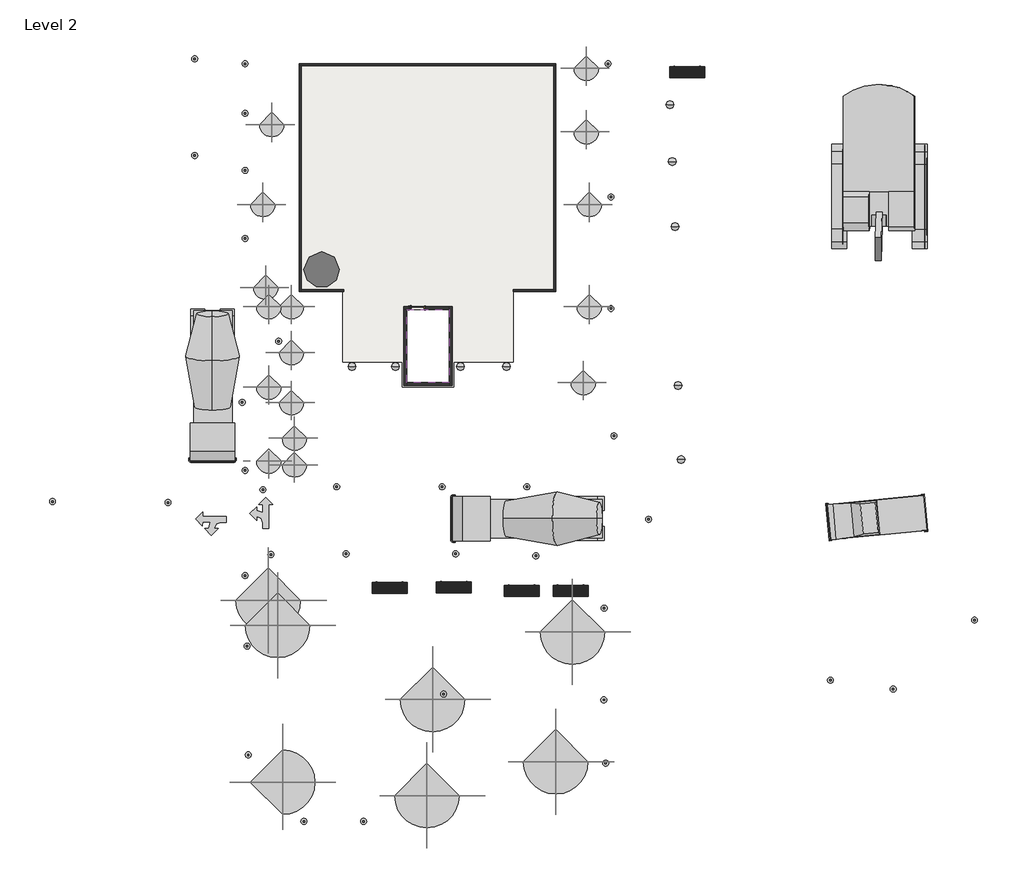
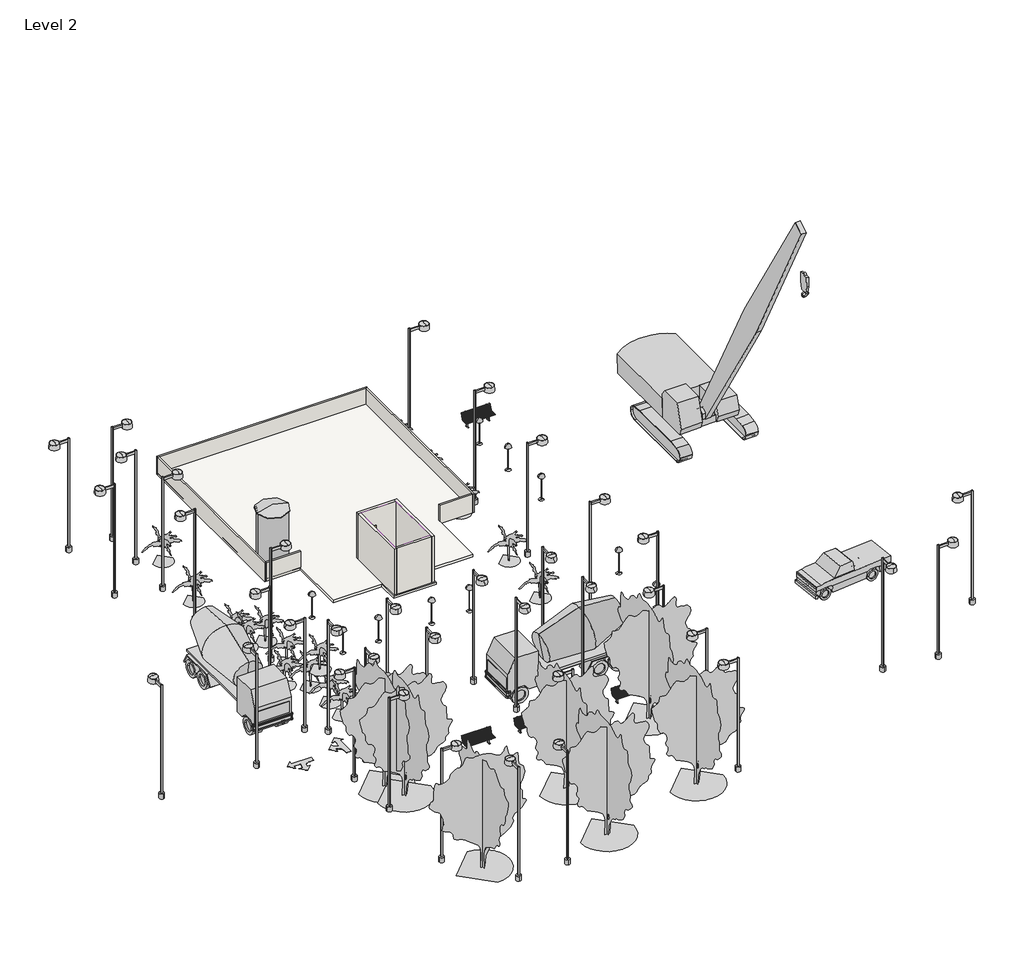
# One storey, incomplete: 46 light fixtures, 34 geographic elements, 9 walls, 1 covering, 1 door, 1 proxy, 1 slab.
"""IFC4 building model written with IfcOpenShell, lengths in millimetres."""

from ifc_helpers import new_model, si_unit, frame, origin, place, context, project, spatial, polyline, outline, extrude, faceted_brep, transform, mapped, element, save
from components import m_watertank_water_tank_eee2c874, door_ef1582a9, geographic_element_33b6fea6, m_concrete_truck_concrete_truck_8dc9909d, m_construction_crane_c1d51077, m_park_bench_1800mm_81f1f144, m_rpc_tree_tropical_australian_tree_fern_1_8_meters_0203a3dd, m_truck_pick_up_pick_up_truck_f485962c, rpc_tree_deciduous_honey_locust_25_cc46a1f1, m_floor_lamp_hemispheric_100w_277v_4a08ccbb, m_street_light_standard_400w_halogen_120v_204dbcbb

model = new_model("IFC4")

# Units and contexts
model_context = context("Model", 3, world=origin())
ifc_project = project(units=[si_unit("LENGTHUNIT", "METRE", prefix="MILLI")], contexts=[model_context])

# Site, building, storey
site = spatial("IfcSite", under=ifc_project)
building = spatial("IfcBuilding", under=site)
storey = spatial("IfcBuildingStorey", under=building, Name="Level 2", Elevation=3200.4)

# Proxy
placement = place(None, origin())
m_watertank_water_tank_shape = m_watertank_water_tank_eee2c874(model_context)
element("IfcBuildingElementProxy", 1, Name="M_WaterTank : Water Tank", ObjectType="M_WaterTank : Water Tank", at=placement, inside=storey, context=model_context, shape_type="MappedRepresentation", body=[
    mapped(m_watertank_water_tank_shape, transform((-12398.6299582, 9055.036641, 3352.8), x_axis=(1.0, 0.0, 0.0), y_axis=(0.0, 1.0, 0.0), z_axis=(0.0, 0.0, 1.0))),
])

# Covering
element("IfcCovering", 2, ObjectType="2' x 4' ACT System", at=placement, inside=storey, context=model_context, shape_type="SweptSolid", body=[
    extrude(outline(polyline([(-8032.1581554, 6997.036641), (-5822.3581554, 6997.036641), (-5822.3581554, 3237.836641), (-8032.1581554, 3237.836641), (-8032.1581554, 6997.036641)])), frame((0.0, 0.0, 6400.8), z_axis=(0.0, 0.0, 1.0), x_axis=(1.0, 0.0, 0.0)), (0.0, 0.0, 1.0), 57.15),
])

# Door
door_shape = door_ef1582a9(model_context)
element("IfcDoor", 3, ObjectType="M_Door-Interior-Single-6_Panel-Wood : 2'5\"", at=placement, inside=storey, context=model_context, shape_type="MappedRepresentation", body=[
    mapped(door_shape, transform((-7498.7581554, 7076.411641, 3352.8), x_axis=(1.0, 0.0, 0.0), y_axis=(0.0, 1.0, 0.0), z_axis=(0.0, 0.0, 1.0))),
])

# Geographic elements
geographic_element_shape = geographic_element_33b6fea6(model_context)
element("IfcGeographicElement", 4, at=placement, inside=storey, context=model_context, shape_type="MappedRepresentation", body=[
    mapped(geographic_element_shape, transform((-17303.3787549, -3805.4849597, -152.4), x_axis=(0.016862452734669187, 0.9998578187361297, 0.0), y_axis=(-0.9998578187361297, 0.016862452734669187, 0.0), z_axis=(0.0, 0.0, 1.0))),
])
element("IfcGeographicElement", 5, at=placement, inside=storey, context=model_context, shape_type="MappedRepresentation", body=[
    mapped(geographic_element_shape, transform((-15269.4299582, -4255.163359, -152.4), x_axis=(1.0, 0.0, 0.0), y_axis=(0.0, 1.0, 0.0), z_axis=(0.0, 0.0, 1.0))),
])
m_concrete_truck_concrete_truck_shape = m_concrete_truck_concrete_truck_8dc9909d(model_context)
element("IfcGeographicElement", 6, ObjectType="M_Concrete Truck : Concrete Truck", at=placement, inside=storey, context=model_context, shape_type="MappedRepresentation", body=[
    mapped(m_concrete_truck_concrete_truck_shape, transform((-17968.6684197, 3155.7751025, -152.4), x_axis=(1.0, 0.0, 0.0), y_axis=(0.0, 1.0, 0.0), z_axis=(0.0, 0.0, 1.0))),
])
element("IfcGeographicElement", 7, ObjectType="M_Concrete Truck : Concrete Truck", at=placement, inside=storey, context=model_context, shape_type="MappedRepresentation", body=[
    mapped(m_concrete_truck_concrete_truck_shape, transform((-1737.0914966, -3803.8248975, -152.4), x_axis=(0.0, -1.0, 0.0), y_axis=(1.0, 0.0, 0.0), z_axis=(0.0, 0.0, 1.0))),
])
m_construction_crane_shape = m_construction_crane_c1d51077(model_context)
element("IfcGeographicElement", 8, ObjectType="M_Construction Crane", at=placement, inside=storey, context=model_context, shape_type="MappedRepresentation", body=[
    mapped(m_construction_crane_shape, transform((21981.1338705, 15716.0751025, 120.4025575), x_axis=(0.9998666340647555, 0.0, 0.016331383407914204), y_axis=(0.0, 1.0, 0.0), z_axis=(-0.016331383407914204, 0.0, 0.9998666340647555))),
])
m_park_bench_1800mm_shape = m_park_bench_1800mm_81f1f144(model_context)
element("IfcGeographicElement", 9, ObjectType="M_Park Bench : 1800mm", at=placement, inside=storey, context=model_context, shape_type="MappedRepresentation", body=[
    mapped(m_park_bench_1800mm_shape, transform((6396.7700418, 19239.836641, -134.1456114), x_axis=(1.0, 0.0, 0.0), y_axis=(0.0, 1.0, 0.0), z_axis=(0.0, 0.0, 1.0))),
])
element("IfcGeographicElement", 10, ObjectType="M_Park Bench : 1800mm", at=placement, inside=storey, context=model_context, shape_type="MappedRepresentation", body=[
    mapped(m_park_bench_1800mm_shape, transform((402.3700418, -7455.563359, -152.4), x_axis=(1.0, 0.0, 0.0), y_axis=(0.0, 1.0, 0.0), z_axis=(0.0, 0.0, 1.0))),
])
element("IfcGeographicElement", 11, ObjectType="M_Park Bench : 1800mm", at=placement, inside=storey, context=model_context, shape_type="MappedRepresentation", body=[
    mapped(m_park_bench_1800mm_shape, transform((-2112.2299582, -7455.563359, -152.4), x_axis=(1.0, 0.0, 0.0), y_axis=(0.0, 1.0, 0.0), z_axis=(0.0, 0.0, 1.0))),
])
element("IfcGeographicElement", 12, ObjectType="M_Park Bench : 1800mm", at=placement, inside=storey, context=model_context, shape_type="MappedRepresentation", body=[
    mapped(m_park_bench_1800mm_shape, transform((-5593.7581554, -7257.9919216, -152.4), x_axis=(1.0, 0.0, 0.0), y_axis=(0.0, 1.0, 0.0), z_axis=(0.0, 0.0, 1.0))),
])
element("IfcGeographicElement", 13, ObjectType="M_Park Bench : 1800mm", at=placement, inside=storey, context=model_context, shape_type="MappedRepresentation", body=[
    mapped(m_park_bench_1800mm_shape, transform((-8906.7299582, -7303.163359, -152.4), x_axis=(1.0, 0.0, 0.0), y_axis=(0.0, 1.0, 0.0), z_axis=(0.0, 0.0, 1.0))),
])
m_rpc_tree_tropical_australian_tree_fern_1_8_meters_shape = m_rpc_tree_tropical_australian_tree_fern_1_8_meters_0203a3dd(model_context)
element("IfcGeographicElement", 14, ObjectType="M_RPC Tree - Tropical : Australian Tree Fern - 1.8 Meters", at=placement, inside=storey, context=model_context, shape_type="MappedRepresentation", body=[
    mapped(m_rpc_tree_tropical_australian_tree_fern_1_8_meters_shape, transform((1214.9733707, 19417.636641, -152.4), x_axis=(1.0, 0.0, 0.0), y_axis=(0.0, 1.0, 0.0), z_axis=(0.0, 0.0, 1.0))),
])
element("IfcGeographicElement", 15, ObjectType="M_RPC Tree - Tropical : Australian Tree Fern - 1.8 Meters", at=placement, inside=storey, context=model_context, shape_type="MappedRepresentation", body=[
    mapped(m_rpc_tree_tropical_australian_tree_fern_1_8_meters_shape, transform((1214.9733707, 16141.036641, -152.4), x_axis=(1.0, 0.0, 0.0), y_axis=(0.0, 1.0, 0.0), z_axis=(0.0, 0.0, 1.0))),
])
element("IfcGeographicElement", 16, ObjectType="M_RPC Tree - Tropical : Australian Tree Fern - 1.8 Meters", at=placement, inside=storey, context=model_context, shape_type="MappedRepresentation", body=[
    mapped(m_rpc_tree_tropical_australian_tree_fern_1_8_meters_shape, transform((1367.3733707, 12407.236641, -152.4), x_axis=(1.0, 0.0, 0.0), y_axis=(0.0, 1.0, 0.0), z_axis=(0.0, 0.0, 1.0))),
])
element("IfcGeographicElement", 17, ObjectType="M_RPC Tree - Tropical : Australian Tree Fern - 1.8 Meters", at=placement, inside=storey, context=model_context, shape_type="MappedRepresentation", body=[
    mapped(m_rpc_tree_tropical_australian_tree_fern_1_8_meters_shape, transform((1367.3733707, 7149.436641, -152.4), x_axis=(1.0, 0.0, 0.0), y_axis=(0.0, 1.0, 0.0), z_axis=(0.0, 0.0, 1.0))),
])
element("IfcGeographicElement", 18, ObjectType="M_RPC Tree - Tropical : Australian Tree Fern - 1.8 Meters", at=placement, inside=storey, context=model_context, shape_type="MappedRepresentation", body=[
    mapped(m_rpc_tree_tropical_australian_tree_fern_1_8_meters_shape, transform((1062.5733707, 3237.836641, -152.4), x_axis=(1.0, 0.0, 0.0), y_axis=(0.0, 1.0, 0.0), z_axis=(0.0, 0.0, 1.0))),
])
element("IfcGeographicElement", 19, ObjectType="M_RPC Tree - Tropical : Australian Tree Fern - 1.8 Meters", at=placement, inside=storey, context=model_context, shape_type="MappedRepresentation", body=[
    mapped(m_rpc_tree_tropical_australian_tree_fern_1_8_meters_shape, transform((-15117.2266293, 3009.236641, -152.4), x_axis=(1.0, 0.0, 0.0), y_axis=(0.0, 1.0, 0.0), z_axis=(0.0, 0.0, 1.0))),
])
element("IfcGeographicElement", 20, ObjectType="M_RPC Tree - Tropical : Australian Tree Fern - 1.8 Meters", at=placement, inside=storey, context=model_context, shape_type="MappedRepresentation", body=[
    mapped(m_rpc_tree_tropical_australian_tree_fern_1_8_meters_shape, transform((-15117.2266293, 7149.436641, -152.4), x_axis=(1.0, 0.0, 0.0), y_axis=(0.0, 1.0, 0.0), z_axis=(0.0, 0.0, 1.0))),
])
element("IfcGeographicElement", 21, ObjectType="M_RPC Tree - Tropical : Australian Tree Fern - 1.8 Meters", at=placement, inside=storey, context=model_context, shape_type="MappedRepresentation", body=[
    mapped(m_rpc_tree_tropical_australian_tree_fern_1_8_meters_shape, transform((-14964.8266293, 16522.036641, -152.4), x_axis=(1.0, 0.0, 0.0), y_axis=(0.0, 1.0, 0.0), z_axis=(0.0, 0.0, 1.0))),
])
element("IfcGeographicElement", 22, ObjectType="M_RPC Tree - Tropical : Australian Tree Fern - 1.8 Meters", at=placement, inside=storey, context=model_context, shape_type="MappedRepresentation", body=[
    mapped(m_rpc_tree_tropical_australian_tree_fern_1_8_meters_shape, transform((-15117.2266293, -800.763359, 3200.4), x_axis=(1.0, 0.0, 0.0), y_axis=(0.0, 1.0, 0.0), z_axis=(0.0, 0.0, 1.0))),
])
element("IfcGeographicElement", 23, ObjectType="M_RPC Tree - Tropical : Australian Tree Fern - 1.8 Meters", at=placement, inside=storey, context=model_context, shape_type="MappedRepresentation", body=[
    mapped(m_rpc_tree_tropical_australian_tree_fern_1_8_meters_shape, transform((-15422.0266293, 12407.236641, -152.4), x_axis=(1.0, 0.0, 0.0), y_axis=(0.0, 1.0, 0.0), z_axis=(0.0, 0.0, 1.0))),
])
element("IfcGeographicElement", 24, ObjectType="M_RPC Tree - Tropical : Australian Tree Fern - 1.8 Meters", at=placement, inside=storey, context=model_context, shape_type="MappedRepresentation", body=[
    mapped(m_rpc_tree_tropical_australian_tree_fern_1_8_meters_shape, transform((-15269.6266293, 8140.036641, -152.4), x_axis=(1.0, 0.0, 0.0), y_axis=(0.0, 1.0, 0.0), z_axis=(0.0, 0.0, 1.0))),
])
element("IfcGeographicElement", 25, ObjectType="M_RPC Tree - Tropical : Australian Tree Fern - 1.8 Meters", at=placement, inside=storey, context=model_context, shape_type="MappedRepresentation", body=[
    mapped(m_rpc_tree_tropical_australian_tree_fern_1_8_meters_shape, transform((-13948.8266293, 7149.436641, -152.4), x_axis=(1.0, 0.0, 0.0), y_axis=(0.0, 1.0, 0.0), z_axis=(0.0, 0.0, 1.0))),
])
element("IfcGeographicElement", 26, ObjectType="M_RPC Tree - Tropical : Australian Tree Fern - 1.8 Meters", at=placement, inside=storey, context=model_context, shape_type="MappedRepresentation", body=[
    mapped(m_rpc_tree_tropical_australian_tree_fern_1_8_meters_shape, transform((-13948.8266293, 4787.236641, -152.4), x_axis=(1.0, 0.0, 0.0), y_axis=(0.0, 1.0, 0.0), z_axis=(0.0, 0.0, 1.0))),
])
element("IfcGeographicElement", 27, ObjectType="M_RPC Tree - Tropical : Australian Tree Fern - 1.8 Meters", at=placement, inside=storey, context=model_context, shape_type="MappedRepresentation", body=[
    mapped(m_rpc_tree_tropical_australian_tree_fern_1_8_meters_shape, transform((-13948.8266293, 2209.136641, -152.4), x_axis=(1.0, 0.0, 0.0), y_axis=(0.0, 1.0, 0.0), z_axis=(0.0, 0.0, 1.0))),
])
element("IfcGeographicElement", 28, ObjectType="M_RPC Tree - Tropical : Australian Tree Fern - 1.8 Meters", at=placement, inside=storey, context=model_context, shape_type="MappedRepresentation", body=[
    mapped(m_rpc_tree_tropical_australian_tree_fern_1_8_meters_shape, transform((-13796.4266293, 380.336641, -152.4), x_axis=(1.0, 0.0, 0.0), y_axis=(0.0, 1.0, 0.0), z_axis=(0.0, 0.0, 1.0))),
])
element("IfcGeographicElement", 29, ObjectType="M_RPC Tree - Tropical : Australian Tree Fern - 1.8 Meters", at=placement, inside=storey, context=model_context, shape_type="MappedRepresentation", body=[
    mapped(m_rpc_tree_tropical_australian_tree_fern_1_8_meters_shape, transform((-13796.4266293, -991.263359, -152.4), x_axis=(1.0, 0.0, 0.0), y_axis=(0.0, 1.0, 0.0), z_axis=(0.0, 0.0, 1.0))),
])
m_truck_pick_up_pick_up_truck_shape = m_truck_pick_up_pick_up_truck_f485962c(model_context)
element("IfcGeographicElement", 30, ObjectType="M_Truck - Pick-Up : Pick-Up Truck", at=placement, inside=storey, context=model_context, shape_type="MappedRepresentation", body=[
    mapped(m_truck_pick_up_pick_up_truck_shape, transform((15628.1031197, -3722.1387124, -152.4), x_axis=(0.0952515948864838, -0.9954532302783397, 0.0), y_axis=(0.9954532302783397, 0.0952515948864838, 0.0), z_axis=(0.0, 0.0, 1.0))),
])
rpc_tree_deciduous_honey_locust_25_shape = rpc_tree_deciduous_honey_locust_25_cc46a1f1(model_context)
element("IfcGeographicElement", 31, ObjectType="RPC Tree - Deciduous : Honey Locust - 25'", at=placement, inside=storey, context=model_context, shape_type="MappedRepresentation", body=[
    mapped(rpc_tree_deciduous_honey_locust_25_shape, transform((503.9700418, -9597.0505555, -152.4), x_axis=(1.0, 0.0, 0.0), y_axis=(0.0, 1.0, 0.0), z_axis=(0.0, 0.0, 1.0))),
])
element("IfcGeographicElement", 32, ObjectType="RPC Tree - Deciduous : Honey Locust - 25'", at=placement, inside=storey, context=model_context, shape_type="MappedRepresentation", body=[
    mapped(rpc_tree_deciduous_honey_locust_25_shape, transform((-15145.9347705, -7965.3174698, -152.4), x_axis=(1.0, 0.0, 0.0), y_axis=(0.0, 1.0, 0.0), z_axis=(0.0, 0.0, 1.0))),
])
element("IfcGeographicElement", 33, ObjectType="RPC Tree - Deciduous : Honey Locust - 25'", at=placement, inside=storey, context=model_context, shape_type="MappedRepresentation", body=[
    mapped(rpc_tree_deciduous_honey_locust_25_shape, transform((-6694.0035501, -13068.9779282, -152.4), x_axis=(1.0, 0.0, 0.0), y_axis=(0.0, 1.0, 0.0), z_axis=(0.0, 0.0, 1.0))),
])
element("IfcGeographicElement", 34, ObjectType="RPC Tree - Deciduous : Honey Locust - 25'", at=placement, inside=storey, context=model_context, shape_type="MappedRepresentation", body=[
    mapped(rpc_tree_deciduous_honey_locust_25_shape, transform((-359.6299582, -16269.9199129, -152.4), x_axis=(1.0, 0.0, 0.0), y_axis=(0.0, 1.0, 0.0), z_axis=(0.0, 0.0, 1.0))),
])
element("IfcGeographicElement", 35, ObjectType="RPC Tree - Deciduous : Honey Locust - 25'", at=placement, inside=storey, context=model_context, shape_type="MappedRepresentation", body=[
    mapped(rpc_tree_deciduous_honey_locust_25_shape, transform((-14405.8299582, -17330.8911171, -152.4), x_axis=(0.0, 1.0, 0.0), y_axis=(-1.0, 0.0, 0.0), z_axis=(0.0, 0.0, 1.0))),
])
element("IfcGeographicElement", 36, ObjectType="RPC Tree - Deciduous : Honey Locust - 25'", at=placement, inside=storey, context=model_context, shape_type="MappedRepresentation", body=[
    mapped(rpc_tree_deciduous_honey_locust_25_shape, transform((-14664.2636101, -9251.2975297, -152.4), x_axis=(1.0, 0.0, 0.0), y_axis=(0.0, 1.0, 0.0), z_axis=(0.0, 0.0, 1.0))),
])
element("IfcGeographicElement", 37, ObjectType="RPC Tree - Deciduous : Honey Locust - 25'", at=placement, inside=storey, context=model_context, shape_type="MappedRepresentation", body=[
    mapped(rpc_tree_deciduous_honey_locust_25_shape, transform((-6981.0037801, -18013.7214545, -152.4), x_axis=(1.0, 0.0, 0.0), y_axis=(0.0, 1.0, 0.0), z_axis=(0.0, 0.0, 1.0))),
])

# Light fixtures
m_floor_lamp_hemispheric_100w_277v_shape = m_floor_lamp_hemispheric_100w_277v_4a08ccbb(model_context)
element("IfcLightFixture", 38, ObjectType="M_Floor Lamp - Hemispheric : 100W - 277V", at=placement, inside=storey, context=model_context, shape_type="MappedRepresentation", body=[
    mapped(m_floor_lamp_hemispheric_100w_277v_shape, transform((-8603.6581554, 4063.336641, -152.4), x_axis=(1.0, 0.0, 0.0), y_axis=(0.0, 1.0, 0.0), z_axis=(0.0, 0.0, 1.0))),
])
element("IfcLightFixture", 39, ObjectType="M_Floor Lamp - Hemispheric : 100W - 277V", at=placement, inside=storey, context=model_context, shape_type="MappedRepresentation", body=[
    mapped(m_floor_lamp_hemispheric_100w_277v_shape, transform((-10837.1299582, 4063.336641, -152.4), x_axis=(1.0, 0.0, 0.0), y_axis=(0.0, 1.0, 0.0), z_axis=(0.0, 0.0, 1.0))),
])
element("IfcLightFixture", 40, ObjectType="M_Floor Lamp - Hemispheric : 100W - 277V", at=placement, inside=storey, context=model_context, shape_type="MappedRepresentation", body=[
    mapped(m_floor_lamp_hemispheric_100w_277v_shape, transform((-2899.6299582, 4063.336641, -152.4), x_axis=(1.0, 0.0, 0.0), y_axis=(0.0, 1.0, 0.0), z_axis=(0.0, 0.0, 1.0))),
])
element("IfcLightFixture", 41, ObjectType="M_Floor Lamp - Hemispheric : 100W - 277V", at=placement, inside=storey, context=model_context, shape_type="MappedRepresentation", body=[
    mapped(m_floor_lamp_hemispheric_100w_277v_shape, transform((-5261.8299582, 4063.336641, -152.4), x_axis=(1.0, 0.0, 0.0), y_axis=(0.0, 1.0, 0.0), z_axis=(0.0, 0.0, 1.0))),
])
element("IfcLightFixture", 42, ObjectType="M_Floor Lamp - Hemispheric : 100W - 277V", at=placement, inside=storey, context=model_context, shape_type="MappedRepresentation", body=[
    mapped(m_floor_lamp_hemispheric_100w_277v_shape, transform((-10621.2299582, 7809.836641, -152.4), x_axis=(1.0, 0.0, 0.0), y_axis=(0.0, 1.0, 0.0), z_axis=(0.0, 0.0, 1.0))),
])
element("IfcLightFixture", 43, ObjectType="M_Floor Lamp - Hemispheric : 60W - 120V", at=placement, inside=storey, context=model_context, shape_type="MappedRepresentation", body=[
    mapped(m_floor_lamp_hemispheric_100w_277v_shape, transform((5513.1332848, 17539.0360942, -148.5785469), x_axis=(1.0, 0.0, 0.0), y_axis=(0.0, 1.0, 0.0), z_axis=(0.0, 0.0, 1.0))),
])
element("IfcLightFixture", 44, ObjectType="M_Floor Lamp - Hemispheric : 60W - 120V", at=placement, inside=storey, context=model_context, shape_type="MappedRepresentation", body=[
    mapped(m_floor_lamp_hemispheric_100w_277v_shape, transform((5634.7700418, 14617.036641, -146.5917854), x_axis=(1.0, 0.0, 0.0), y_axis=(0.0, 1.0, 0.0), z_axis=(0.0, 0.0, 1.0))),
])
element("IfcLightFixture", 45, ObjectType="M_Floor Lamp - Hemispheric : 60W - 120V", at=placement, inside=storey, context=model_context, shape_type="MappedRepresentation", body=[
    mapped(m_floor_lamp_hemispheric_100w_277v_shape, transform((5787.1700418, 11264.236641, -144.1025506), x_axis=(1.0, 0.0, 0.0), y_axis=(0.0, 1.0, 0.0), z_axis=(0.0, 0.0, 1.0))),
])
element("IfcLightFixture", 46, ObjectType="M_Floor Lamp - Hemispheric : 60W - 120V", at=placement, inside=storey, context=model_context, shape_type="MappedRepresentation", body=[
    mapped(m_floor_lamp_hemispheric_100w_277v_shape, transform((5939.5700418, 3085.436641, -141.6133158), x_axis=(1.0, 0.0, 0.0), y_axis=(0.0, 1.0, 0.0), z_axis=(0.0, 0.0, 1.0))),
])
element("IfcLightFixture", 47, ObjectType="M_Floor Lamp - Hemispheric : 60W - 120V", at=placement, inside=storey, context=model_context, shape_type="MappedRepresentation", body=[
    mapped(m_floor_lamp_hemispheric_100w_277v_shape, transform((6091.9700418, -724.563359, -145.0919931), x_axis=(1.0, 0.0, 0.0), y_axis=(0.0, 1.0, 0.0), z_axis=(0.0, 0.0, 1.0))),
])
m_street_light_standard_400w_halogen_120v_shape = m_street_light_standard_400w_halogen_120v_204dbcbb(model_context)
element("IfcLightFixture", 48, ObjectType="M_Street Light - Standard : 400W Halogen - 120V", at=placement, inside=storey, context=model_context, shape_type="MappedRepresentation", body=[
    mapped(m_street_light_standard_400w_halogen_120v_shape, transform((2332.7700418, 19646.236641, -152.4), x_axis=(-1.0, 0.0, 0.0), y_axis=(0.0, -1.0, 0.0), z_axis=(0.0, 0.0, 1.0))),
])
element("IfcLightFixture", 49, ObjectType="M_Street Light - Standard : 400W Halogen - 120V", at=placement, inside=storey, context=model_context, shape_type="MappedRepresentation", body=[
    mapped(m_street_light_standard_400w_halogen_120v_shape, transform((2485.1700418, 12788.236641, -152.4), x_axis=(-1.0, 0.0, 0.0), y_axis=(0.0, -1.0, 0.0), z_axis=(0.0, 0.0, 1.0))),
])
element("IfcLightFixture", 50, ObjectType="M_Street Light - Standard : 400W Halogen - 120V", at=placement, inside=storey, context=model_context, shape_type="MappedRepresentation", body=[
    mapped(m_street_light_standard_400w_halogen_120v_shape, transform((2637.5700418, 494.636641, -152.4), x_axis=(-1.0, 0.0, 0.0), y_axis=(0.0, -1.0, 0.0), z_axis=(0.0, 0.0, 1.0))),
])
element("IfcLightFixture", 51, ObjectType="M_Street Light - Standard : 400W Halogen - 120V", at=placement, inside=storey, context=model_context, shape_type="MappedRepresentation", body=[
    mapped(m_street_light_standard_400w_halogen_120v_shape, transform((2485.1700418, 7047.836641, -152.4), x_axis=(-1.0, 0.0, 0.0), y_axis=(0.0, -1.0, 0.0), z_axis=(0.0, 0.0, 1.0))),
])
element("IfcLightFixture", 52, ObjectType="M_Street Light - Standard : 400W Halogen - 120V", at=placement, inside=storey, context=model_context, shape_type="MappedRepresentation", body=[
    mapped(m_street_light_standard_400w_halogen_120v_shape, transform((-15421.8299582, -2273.963359, 0.0), x_axis=(0.0, 1.0, 0.0), y_axis=(-1.0, 0.0, 0.0), z_axis=(0.0, 0.0, 1.0))),
])
element("IfcLightFixture", 53, ObjectType="M_Street Light - Standard : 400W Halogen - 120V", at=placement, inside=storey, context=model_context, shape_type="MappedRepresentation", body=[
    mapped(m_street_light_standard_400w_halogen_120v_shape, transform((-11624.5299582, -2121.563359, 0.0), x_axis=(0.0, 1.0, 0.0), y_axis=(-1.0, 0.0, 0.0), z_axis=(0.0, 0.0, 1.0))),
])
element("IfcLightFixture", 54, ObjectType="M_Street Light - Standard : 400W Halogen - 120V", at=placement, inside=storey, context=model_context, shape_type="MappedRepresentation", body=[
    mapped(m_street_light_standard_400w_halogen_120v_shape, transform((-6203.3581554, -2121.563359, 0.0), x_axis=(0.0, 1.0, 0.0), y_axis=(-1.0, 0.0, 0.0), z_axis=(0.0, 0.0, 1.0))),
])
element("IfcLightFixture", 55, ObjectType="M_Street Light - Standard : 400W Halogen - 120V", at=placement, inside=storey, context=model_context, shape_type="MappedRepresentation", body=[
    mapped(m_street_light_standard_400w_halogen_120v_shape, transform((-1845.5299582, -2121.563359, 0.0), x_axis=(0.0, 1.0, 0.0), y_axis=(-1.0, 0.0, 0.0), z_axis=(0.0, 0.0, 1.0))),
])
element("IfcLightFixture", 56, ObjectType="M_Street Light - Standard : 400W Halogen - 120V", at=placement, inside=storey, context=model_context, shape_type="MappedRepresentation", body=[
    mapped(m_street_light_standard_400w_halogen_120v_shape, transform((-15006.5505126, -5608.7033445, 0.0), x_axis=(0.0, 1.0, 0.0), y_axis=(-1.0, 0.0, 0.0), z_axis=(0.0, 0.0, 1.0))),
])
element("IfcLightFixture", 57, ObjectType="M_Street Light - Standard : 400W Halogen - 120V", at=placement, inside=storey, context=model_context, shape_type="MappedRepresentation", body=[
    mapped(m_street_light_standard_400w_halogen_120v_shape, transform((-11141.9299582, -5575.963359, 0.0), x_axis=(0.0, 1.0, 0.0), y_axis=(-1.0, 0.0, 0.0), z_axis=(0.0, 0.0, 1.0))),
])
element("IfcLightFixture", 58, ObjectType="M_Street Light - Standard : 400W Halogen - 120V", at=placement, inside=storey, context=model_context, shape_type="MappedRepresentation", body=[
    mapped(m_street_light_standard_400w_halogen_120v_shape, transform((-5503.1299582, -5575.963359, 0.0), x_axis=(0.0, 1.0, 0.0), y_axis=(-1.0, 0.0, 0.0), z_axis=(0.0, 0.0, 1.0))),
])
element("IfcLightFixture", 59, ObjectType="M_Street Light - Standard : 400W Halogen - 120V", at=placement, inside=storey, context=model_context, shape_type="MappedRepresentation", body=[
    mapped(m_street_light_standard_400w_halogen_120v_shape, transform((-1383.290395, -5679.9051322, 0.0), x_axis=(0.0, 1.0, 0.0), y_axis=(-1.0, 0.0, 0.0), z_axis=(0.0, 0.0, 1.0))),
])
element("IfcLightFixture", 60, ObjectType="M_Street Light - Standard : 400W Halogen - 120V", at=placement, inside=storey, context=model_context, shape_type="MappedRepresentation", body=[
    mapped(m_street_light_standard_400w_halogen_120v_shape, transform((2129.5700418, -8369.963359, -152.4), x_axis=(1.0, 0.0, 0.0), y_axis=(0.0, 1.0, 0.0), z_axis=(0.0, 0.0, 1.0))),
])
element("IfcLightFixture", 61, ObjectType="M_Street Light - Standard : 400W Halogen - 120V", at=placement, inside=storey, context=model_context, shape_type="MappedRepresentation", body=[
    mapped(m_street_light_standard_400w_halogen_120v_shape, transform((2117.2753399, -13089.3237573, -152.4), x_axis=(1.0, 0.0, 0.0), y_axis=(0.0, 1.0, 0.0), z_axis=(0.0, 0.0, 1.0))),
])
element("IfcLightFixture", 62, ObjectType="M_Street Light - Standard : 400W Halogen - 120V", at=placement, inside=storey, context=model_context, shape_type="MappedRepresentation", body=[
    mapped(m_street_light_standard_400w_halogen_120v_shape, transform((2210.8272988, -16350.1092884, -152.4), x_axis=(1.0, 0.0, 0.0), y_axis=(0.0, 1.0, 0.0), z_axis=(0.0, 0.0, 1.0))),
])
element("IfcLightFixture", 63, ObjectType="M_Street Light - Standard : 400W Halogen - 120V", at=placement, inside=storey, context=model_context, shape_type="MappedRepresentation", body=[
    mapped(m_street_light_standard_400w_halogen_120v_shape, transform((13769.7128986, -12075.4373856, -152.4), x_axis=(0.0, 1.0, 0.0), y_axis=(-1.0, 0.0, 0.0), z_axis=(0.0, 0.0, 1.0))),
])
element("IfcLightFixture", 64, ObjectType="M_Street Light - Standard : 400W Halogen - 120V", at=placement, inside=storey, context=model_context, shape_type="MappedRepresentation", body=[
    mapped(m_street_light_standard_400w_halogen_120v_shape, transform((16994.3658729, -12532.6373856, -152.4), x_axis=(-1.0, 0.0, 0.0), y_axis=(0.0, -1.0, 0.0), z_axis=(0.0, 0.0, 1.0))),
])
element("IfcLightFixture", 65, ObjectType="M_Street Light - Standard : 400W Halogen - 120V", at=placement, inside=storey, context=model_context, shape_type="MappedRepresentation", body=[
    mapped(m_street_light_standard_400w_halogen_120v_shape, transform((21179.5700418, -8979.563359, -152.4), x_axis=(1.0, 0.0, 0.0), y_axis=(0.0, 1.0, 0.0), z_axis=(0.0, 0.0, 1.0))),
])
element("IfcLightFixture", 66, ObjectType="M_Street Light - Standard : 400W Halogen - 120V", at=placement, inside=storey, context=model_context, shape_type="MappedRepresentation", body=[
    mapped(m_street_light_standard_400w_halogen_120v_shape, transform((4415.5700418, -3797.963359, -152.4), x_axis=(1.0, 0.0, 0.0), y_axis=(0.0, 1.0, 0.0), z_axis=(0.0, 0.0, 1.0))),
])
element("IfcLightFixture", 67, ObjectType="M_Street Light - Standard : 400W Halogen - 120V", at=placement, inside=storey, context=model_context, shape_type="MappedRepresentation", body=[
    mapped(m_street_light_standard_400w_halogen_120v_shape, transform((-16232.9652381, -10322.7398887, 0.0), x_axis=(-1.0, 0.0, 0.0), y_axis=(0.0, -1.0, 0.0), z_axis=(0.0, 0.0, 1.0))),
])
element("IfcLightFixture", 68, ObjectType="M_Street Light - Standard : 400W Halogen - 120V", at=placement, inside=storey, context=model_context, shape_type="MappedRepresentation", body=[
    mapped(m_street_light_standard_400w_halogen_120v_shape, transform((-16172.8526522, -15918.8024863, 0.0), x_axis=(-1.0, 0.0, 0.0), y_axis=(0.0, -1.0, 0.0), z_axis=(0.0, 0.0, 1.0))),
])
element("IfcLightFixture", 69, ObjectType="M_Street Light - Standard : 400W Halogen - 120V", at=placement, inside=storey, context=model_context, shape_type="MappedRepresentation", body=[
    mapped(m_street_light_standard_400w_halogen_120v_shape, transform((-16336.2299582, 19646.236641, -152.4), x_axis=(-1.0, 0.0, 0.0), y_axis=(0.0, -1.0, 0.0), z_axis=(0.0, 0.0, 1.0))),
])
element("IfcLightFixture", 70, ObjectType="M_Street Light - Standard : 400W Halogen - 120V", at=placement, inside=storey, context=model_context, shape_type="MappedRepresentation", body=[
    mapped(m_street_light_standard_400w_halogen_120v_shape, transform((-16336.2299582, 17093.536641, -152.4), x_axis=(1.0, 0.0, 0.0), y_axis=(0.0, 1.0, 0.0), z_axis=(0.0, 0.0, 1.0))),
])
element("IfcLightFixture", 71, ObjectType="M_Street Light - Standard : 400W Halogen - 120V", at=placement, inside=storey, context=model_context, shape_type="MappedRepresentation", body=[
    mapped(m_street_light_standard_400w_halogen_120v_shape, transform((-16336.2299582, 14159.836641, -152.4), x_axis=(-1.0, 0.0, 0.0), y_axis=(0.0, -1.0, 0.0), z_axis=(0.0, 0.0, 1.0))),
])
element("IfcLightFixture", 72, ObjectType="M_Street Light - Standard : 400W Halogen - 120V", at=placement, inside=storey, context=model_context, shape_type="MappedRepresentation", body=[
    mapped(m_street_light_standard_400w_halogen_120v_shape, transform((-16336.2299582, 10654.636641, -152.4), x_axis=(1.0, 0.0, 0.0), y_axis=(0.0, 1.0, 0.0), z_axis=(0.0, 0.0, 1.0))),
])
element("IfcLightFixture", 73, ObjectType="M_Street Light - Standard : 400W Halogen - 120V", at=placement, inside=storey, context=model_context, shape_type="MappedRepresentation", body=[
    mapped(m_street_light_standard_400w_halogen_120v_shape, transform((-18927.0299582, 19900.236641, -152.3997054), x_axis=(1.0, 0.0, 0.0), y_axis=(0.0, 1.0, 0.0), z_axis=(0.0, 0.0, 1.0))),
])
element("IfcLightFixture", 74, ObjectType="M_Street Light - Standard : 400W Halogen - 120V", at=placement, inside=storey, context=model_context, shape_type="MappedRepresentation", body=[
    mapped(m_street_light_standard_400w_halogen_120v_shape, transform((-18927.0299582, 14921.836641, -152.3997054), x_axis=(1.0, 0.0, 0.0), y_axis=(0.0, 1.0, 0.0), z_axis=(0.0, 0.0, 1.0))),
])
element("IfcLightFixture", 75, ObjectType="M_Street Light - Standard : 400W Halogen - 120V", at=placement, inside=storey, context=model_context, shape_type="MappedRepresentation", body=[
    mapped(m_street_light_standard_400w_halogen_120v_shape, transform((-26242.2299582, -2883.563359, -152.4), x_axis=(0.0, -1.0, 0.0), y_axis=(1.0, 0.0, 0.0), z_axis=(0.0, 0.0, 1.0))),
])
element("IfcLightFixture", 76, ObjectType="M_Street Light - Standard : 400W Halogen - 120V", at=placement, inside=storey, context=model_context, shape_type="MappedRepresentation", body=[
    mapped(m_street_light_standard_400w_halogen_120v_shape, transform((-20298.6299582, -2934.363359, -152.3997054), x_axis=(0.0, -1.0, 0.0), y_axis=(1.0, 0.0, 0.0), z_axis=(0.0, 0.0, 1.0))),
])
element("IfcLightFixture", 77, ObjectType="M_Street Light - Standard : 400W Halogen - 480V", at=placement, inside=storey, context=model_context, shape_type="MappedRepresentation", body=[
    mapped(m_street_light_standard_400w_halogen_120v_shape, transform((-16336.2299582, -6693.563359, -152.4), x_axis=(1.0, 0.0, 0.0), y_axis=(0.0, 1.0, 0.0), z_axis=(0.0, 0.0, 1.0))),
])
element("IfcLightFixture", 78, ObjectType="M_Street Light - Standard : 400W Halogen - 480V", at=placement, inside=storey, context=model_context, shape_type="MappedRepresentation", body=[
    mapped(m_street_light_standard_400w_halogen_120v_shape, transform((-10240.2299582, -19342.763359, -152.4), x_axis=(0.0, -1.0, 0.0), y_axis=(1.0, 0.0, 0.0), z_axis=(0.0, 0.0, 1.0))),
])
element("IfcLightFixture", 79, ObjectType="M_Street Light - Standard : 400W Halogen - 480V", at=placement, inside=storey, context=model_context, shape_type="MappedRepresentation", body=[
    mapped(m_street_light_standard_400w_halogen_120v_shape, transform((-13313.6299582, -19342.763359, -152.4), x_axis=(0.0, -1.0, 0.0), y_axis=(1.0, 0.0, 0.0), z_axis=(0.0, 0.0, 1.0))),
])
element("IfcLightFixture", 80, ObjectType="M_Street Light - Standard : 400W Halogen - 480V", at=placement, inside=storey, context=model_context, shape_type="MappedRepresentation", body=[
    mapped(m_street_light_standard_400w_halogen_120v_shape, transform((-6125.4299582, -12789.563359, -152.4), x_axis=(1.0, 0.0, 0.0), y_axis=(0.0, 1.0, 0.0), z_axis=(0.0, 0.0, 1.0))),
])
element("IfcLightFixture", 81, ObjectType="M_Street Light - Standard : 400W Halogen - 480V", at=placement, inside=storey, context=model_context, shape_type="MappedRepresentation", body=[
    mapped(m_street_light_standard_400w_halogen_120v_shape, transform((-16336.2299582, -1283.363359, -152.4), x_axis=(1.0, 0.0, 0.0), y_axis=(0.0, 1.0, 0.0), z_axis=(0.0, 0.0, 1.0))),
])
element("IfcLightFixture", 82, ObjectType="M_Street Light - Standard : 400W Halogen - 480V", at=placement, inside=storey, context=model_context, shape_type="MappedRepresentation", body=[
    mapped(m_street_light_standard_400w_halogen_120v_shape, transform((-16488.6299582, 2221.836641, -152.4), x_axis=(1.0, 0.0, 0.0), y_axis=(0.0, 1.0, 0.0), z_axis=(0.0, 0.0, 1.0))),
])
element("IfcLightFixture", 83, ObjectType="M_Street Light - Standard : 400W Halogen - 480V", at=placement, inside=storey, context=model_context, shape_type="MappedRepresentation", body=[
    mapped(m_street_light_standard_400w_halogen_120v_shape, transform((-14609.0299582, 5371.436641, -152.4), x_axis=(-1.0, 0.0, 0.0), y_axis=(0.0, -1.0, 0.0), z_axis=(0.0, 0.0, 1.0))),
])

# Slab
element("IfcSlab", 84, ObjectType="Generic - 6\"", at=placement, inside=storey, context=model_context, shape_type="SweptSolid", body=[
    extrude(outline(polyline([(-13542.2299582, 19646.236641), (-359.6299582, 19646.236641), (-359.6299582, 7911.436641), (-2545.7581554, 7911.436641), (-2545.7581554, 4304.636641), (-5593.7581554, 4304.636641), (-5593.7581554, 3015.586641), (-8260.7581554, 3015.586641), (-8260.7581554, 4304.636641), (-11308.7581554, 4304.636641), (-11308.7581554, 7911.436641), (-13542.2299582, 7911.436641), (-13542.2299582, 19646.236641)]), holes=[polyline([(-8032.1581554, 3237.836641), (-5822.3581554, 3237.836641), (-5822.3581554, 6997.036641), (-8032.1581554, 6997.036641), (-8032.1581554, 3237.836641)])]), frame((0.0, 0.0, 3200.4), z_axis=(0.0, 0.0, 1.0), x_axis=(1.0, 0.0, 0.0)), (0.0, 0.0, 1.0), 152.4),
])

# Walls
element("IfcWall", 85, ObjectType="Generic - 4\"", at=placement, inside=storey, context=model_context, shape_type="Brep", body=[
    faceted_brep([(-359.6299582, 19646.236641, 3200.4), (-13542.2299582, 19646.236641, 3200.4), (-13542.2299582, 19646.236641, 4419.6), (-359.6299582, 19646.236641, 4419.6), (-359.6299582, 19544.636641, 3200.4), (-359.6299582, 19544.636641, 4419.6), (-461.2299582, 19544.636641, 4419.6), (-13440.6299582, 19544.636641, 4419.6), (-13542.2299582, 19544.636641, 4419.6), (-13542.2299582, 19544.636641, 3200.4), (-13440.6299582, 19544.636641, 3200.4), (-461.2299582, 19544.636641, 3200.4)], [[[0, 1, 2, 3]], [[4, 5, 6, 7, 8, 9, 10, 11]], [[1, 0, 4, 11, 10, 9]], [[3, 2, 8, 7, 6, 5]], [[2, 1, 9, 8]], [[0, 3, 5, 4]]]),
])
element("IfcWall", 86, ObjectType="Generic - 4\"", at=placement, inside=storey, context=model_context, shape_type="Brep", body=[
    faceted_brep([(-13542.2299582, 19544.636641, 3200.4), (-13542.2299582, 7911.436641, 3200.4), (-13542.2299582, 7911.436641, 4419.6), (-13542.2299582, 19544.636641, 4419.6), (-13440.6299582, 19544.636641, 3200.4), (-13440.6299582, 19544.636641, 4419.6), (-13440.6299582, 8013.036641, 4419.6), (-13440.6299582, 7911.436641, 4419.6), (-13440.6299582, 7911.436641, 3200.4), (-13440.6299582, 8013.036641, 3200.4)], [[[0, 1, 2, 3]], [[4, 5, 6, 7, 8, 9]], [[1, 0, 4, 9, 8]], [[3, 2, 7, 6, 5]], [[0, 3, 5, 4]], [[2, 1, 8, 7]]]),
])
element("IfcWall", 87, ObjectType="Generic - 4\"", at=placement, inside=storey, context=model_context, shape_type="SweptSolid", body=[
    extrude(outline(polyline([(-11257.9581554, 7911.436641), (-13440.6299582, 7911.436641), (-13440.6299582, 8013.036641), (-11257.9581554, 8013.036641), (-11257.9581554, 7911.436641)])), frame((0.0, 0.0, 3200.4), z_axis=(0.0, 0.0, 1.0), x_axis=(1.0, 0.0, 0.0)), (0.0, 0.0, 1.0), 1219.2),
])
element("IfcWall", 88, ObjectType="Generic - 4\"", at=placement, inside=storey, context=model_context, shape_type="Brep", body=[
    faceted_brep([(-359.6299582, 7911.436641, 3200.4), (-359.6299582, 19544.636641, 3200.4), (-359.6299582, 19544.636641, 4419.6), (-359.6299582, 7911.436641, 4419.6), (-461.2299582, 7911.436641, 3200.4), (-461.2299582, 7911.436641, 4419.6), (-461.2299582, 8013.036641, 4419.6), (-461.2299582, 19544.636641, 4419.6), (-461.2299582, 19544.636641, 3200.4), (-461.2299582, 8013.036641, 3200.4)], [[[0, 1, 2, 3]], [[4, 5, 6, 7, 8, 9]], [[1, 0, 4, 9, 8]], [[3, 2, 7, 6, 5]], [[2, 1, 8, 7]], [[0, 3, 5, 4]]]),
])
element("IfcWall", 89, ObjectType="Generic - 4\"", at=placement, inside=storey, context=model_context, shape_type="SweptSolid", body=[
    extrude(outline(polyline([(-461.2299582, 7911.436641), (-2545.7581554, 7911.436641), (-2545.7581554, 8013.036641), (-461.2299582, 8013.036641), (-461.2299582, 7911.436641)])), frame((0.0, 0.0, 3200.4), z_axis=(0.0, 0.0, 1.0), x_axis=(1.0, 0.0, 0.0)), (0.0, 0.0, 1.0), 1219.2),
])
element("IfcWall", 90, ObjectType="Generic - 6\"", at=placement, inside=storey, context=model_context, shape_type="Brep", body=[
    faceted_brep([(-5669.9581554, 3085.436641, 3200.4), (-5669.9581554, 7149.436641, 3200.4), (-5669.9581554, 7149.436641, 6400.8), (-5669.9581554, 3085.436641, 6400.8), (-5822.3581554, 3085.436641, 3200.4), (-5822.3581554, 3085.436641, 6400.8), (-5822.3581554, 3237.836641, 6400.8), (-5822.3581554, 6997.036641, 6400.8), (-5822.3581554, 7149.436641, 6400.8), (-5822.3581554, 7149.436641, 3200.4), (-5822.3581554, 6997.036641, 3200.4), (-5822.3581554, 3237.836641, 3200.4)], [[[0, 1, 2, 3]], [[4, 5, 6, 7, 8, 9, 10, 11]], [[1, 0, 4, 11, 10, 9]], [[3, 2, 8, 7, 6, 5]], [[2, 1, 9, 8]], [[0, 3, 5, 4]]]),
])
element("IfcWall", 91, ObjectType="Generic - 6\"", at=placement, inside=storey, context=model_context, shape_type="Brep", body=[
    faceted_brep([(-5822.3581554, 7149.436641, 3200.4), (-8184.5581554, 7149.436641, 3200.4), (-8184.5581554, 7149.436641, 6400.8), (-5822.3581554, 7149.436641, 6400.8), (-7098.7581554, 7149.436641, 3352.8), (-7098.7581554, 7149.436641, 5206.6), (-7898.7581554, 7149.436641, 5206.6), (-7898.7581554, 7149.436641, 3352.8), (-8184.5581554, 6997.036641, 3200.4), (-8032.1581554, 6997.036641, 3200.4), (-5822.3581554, 6997.036641, 3200.4), (-5822.3581554, 6997.036641, 6400.8), (-8032.1581554, 6997.036641, 6400.8), (-8184.5581554, 6997.036641, 6400.8), (-7098.7581554, 6997.036641, 5206.6), (-7098.7581554, 6997.036641, 3352.8), (-7898.7581554, 6997.036641, 3352.8), (-7898.7581554, 6997.036641, 5206.6)], [[[0, 1, 2, 3], [4, 5, 6, 7]], [[8, 9, 10, 11, 12, 13], [14, 15, 16, 17]], [[1, 0, 10, 9, 8]], [[3, 2, 13, 12, 11]], [[0, 3, 11, 10]], [[2, 1, 8, 13]], [[4, 15, 14, 5]], [[5, 14, 17, 6]], [[6, 17, 16, 7]], [[15, 4, 7, 16]]]),
])
element("IfcWall", 92, ObjectType="Generic - 6\"", at=placement, inside=storey, context=model_context, shape_type="Brep", body=[
    faceted_brep([(-8184.5581554, 6997.036641, 3200.4), (-8184.5581554, 3085.436641, 3200.4), (-8184.5581554, 3085.436641, 6400.8), (-8184.5581554, 6997.036641, 6400.8), (-8032.1581554, 6997.036641, 3200.4), (-8032.1581554, 6997.036641, 6400.8), (-8032.1581554, 3237.836641, 6400.8), (-8032.1581554, 3085.436641, 6400.8), (-8032.1581554, 3085.436641, 3200.4), (-8032.1581554, 3237.836641, 3200.4)], [[[0, 1, 2, 3]], [[4, 5, 6, 7, 8, 9]], [[1, 0, 4, 9, 8]], [[3, 2, 7, 6, 5]], [[0, 3, 5, 4]], [[2, 1, 8, 7]]]),
])
element("IfcWall", 93, ObjectType="Generic - 6\"", at=placement, inside=storey, context=model_context, shape_type="SweptSolid", body=[
    extrude(outline(polyline([(-5822.3581554, 3085.436641), (-8032.1581554, 3085.436641), (-8032.1581554, 3237.836641), (-5822.3581554, 3237.836641), (-5822.3581554, 3085.436641)])), frame((0.0, 0.0, 3200.4), z_axis=(0.0, 0.0, 1.0), x_axis=(1.0, 0.0, 0.0)), (0.0, 0.0, 1.0), 3200.4),
])

save(model, "model.ifc")

# Revit data of these elements
# Type "M_WaterTank : Water Tank"
#   Width Of Top = 3' - 2.97638"
#   Radius = 3' - 0.02362"
#   Height = 11' - 9.73228"
#   Default Elevation = 0
# Type "2' x 4' ACT System"
#   Assembly Code = "C3030210"
#   built-in parameter 1002203 = 1 (stored number, unit not read)
#   built-in parameter 1002202 = 1 (stored number, unit not read)
#   Layers, outside or top first: 0' - 1 5/8" "Default" (function 1); 0' - 0 5/8" "Acoustic Ceiling Tile 24 x 48" (function 5)
# Type "M_Door-Interior-Single-6_Panel-Wood : 2'5\""
#   Type Mark = "11"
#   Assembly Code = "C1020300"
#   Analytic Construction = "Wooden"
#   Top Rail = 0' - 4.72441"
#   Top Panel = 0' - 7.77559"
#   Thickness = 0' - 1.37795"
#   Thermal Resistance (R) = 2.5876 (h·ft²·°F)/BTU
#   Swing Angle [instance default] = 90.00°
#   Stiles = 0' - 4.72441"
#   Rough Width = 2' - 7.49606"
#   Rough Height = 6' - 0.98425"
#   Mullion = 0' - 4.52756"
#   Lock Rail = 0' - 7.87402"
#   Intermediate Rail = 0' - 4.52756"
#   Height = 6' - 0"
#   Width = 2' - 5.52756"
#   Heat Transfer Coefficient (U) = 0.3865 BTU/(h·ft²·°F)
#   Bottom Rail = 0' - 9.05512"
#   Trim Material = Cherry
#   Panel Material = Cherry
#   Frame Material = Cherry
#   Door Handle Material = Aluminum
#   Visual Light Transmittance = 0
#   Solar Heat Gain Coefficient = 0
#   Wall Closure = (empty or 0)
#   Function = (empty or 0)
# Type "M_Concrete Truck : Concrete Truck"
#   Cab Material = Metal, Paint Finish, White, Matte
#   Tire Material = Plastic, Opaque Black
#   Trailer Material = Metal, Paint Finish, White, Matte
# Type "M_Construction Crane"
#   Boom Angle = 60.00°
#   Boom Half = 36' - 1.07087"
#   Boom Length = 72' - 2.14173"
#   Cab Width = 11' - 11.70079"
#   Counter Weight = 18' - 0.53543"
#   Hook = 30.00°
#   Turning Radius = 19' - 0.54333"
#   Width = 16' - 0.91339"
# Type "M_Park Bench : 1800mm"
#   Length = 5' - 10.86614"
#   Seat Material = Wood - Teak
#   Frame Material = Steel, Paint Finish, Dark Gray, Matte
# Type "M_RPC Tree - Tropical : Australian Tree Fern - 1.8 Meters"
#   built-in parameter 1005198 = "{2, 15},{39, RPC-16-FVCN-UWG0-AP53-A000-ST1L-LVER-AU},{1, 0},{1, 0},{2, 35},{1, 8},{5, Color},{1, 0},{1, 0},{3, 0.8},{3, 0.8},{3, 0.8},{1, 8},{7, BBoxMin},{1, 0},{1, 0},{1, 0},{1, 0},{1, 0},{1, 8},{7, BBoxMax},{1, 0},{1, 0},{1, 0},{1, 0},{1, 0},{2, 11},{9, RPCTypeId},{1, 0},{1, 0},{39, RPC-16-FVCN-UWG0-AP53-A000-ST1L-LVER-AU},{1, 6},{14, RPCPlantHeight},{1, 0},{1, 0},{7, 5.90551},{2, 11},{7, keyword},{1, 0},{1, 0},{99, :Geometry:RPC:Australian Tree Fern:Alsophila cooperi (Cyathea australis):Sydney:Tree fern:Tropical.},{2, 11},{8, category},{1, 0},{1, 0},{17, :Trees [Tropical]},{2, 11},{12, LocalizedUID},{1, 0},{1, 0},{20, Australian Tree Fern},{2, 14},{6, Height},{1, 0},{1, 0},{7, 5.90551},{1, 2},{16, Cast Reflections},{1, 0},{1, 0},{1, 0},{1, 2},{12, Cast Shadows},{1, 0},{1, 0},{1, 1},{1, 2},{9, Lock View},{1, 0},{1, 0},{1, 0},{1, 4},{5, ViewC},{1, 0},{1, 0},{1, 0},{2, 11},{20, AdvancedUIDefinition},{1, 0},{1, 0},{0, },{2, 11},{10, AssetLibID},{1, 0},{1, 0},{36, 4D3F6E72-3F99-4203-98E9-AF80B3C7A7A4},{2, 11},{10, BaseSchema},{1, 0},{1, 0},{9, RPCSchema},{2, 11},{12, ExchangeGUID},{1, 0},{1, 0},{0, },{1, 2},{6, Hidden},{1, 0},{1, 0},{1, 0},{1, 4},{11, RPCCategory},{1, 0},{1, 0},{1, 0},{2, 11},{8, RPCImage},{1, 0},{1, 0},{0, },{1, 4},{13, SchemaVersion},{1, 0},{1, 0},{1, 4},{2, 11},{12, UIDefinition},{1, 0},{1, 0},{0, },{2, 11},{6, UIName},{1, 0},{1, 0},{39, RPC-16-FVCN-UWG0-AP53-A000-ST1L-LVER-AU},{2, 11},{11, VersionGUID},{1, 0},{1, 0},{9, RPCSchema},{2, 11},{9, assettype},{1, 0},{1, 0},{11, RPCGeometry},{2, 11},{11, description},{1, 0},{1, 0},{0, },{2, 11},{9, localname},{1, 0},{1, 0},{3, RPC},{2, 11},{9, localtype},{1, 0},{1, 0},{3, RPC},{1, 4},{8, revision},{1, 0},{1, 0},{1, 1},{2, 11},{9, thumbnail},{1, 0},{1, 0},{0, },{1, 4},{7, version},{1, 0},{1, 0},{1, 1},{1, 2},{20, RPC_Cast Reflections},{1, 0},{1, 0},{1, 1},{1, 2},{16, RPC_Cast Shadows},{1, 0},{1, 0},{1, 1},{1, 2},{13, RPC_Lock View},{1, 0},{1, 0},{1, 0},{1, 4},{9, RPC_ViewC},{1, 0},{1, 0},{1, 0},{21, assetlibrary_base.fbx},{1, 5},"
#   built-in parameter 1005195 = "RPC-16-FVCN-UWG0-AP53-A000-ST1L-LVER-AU"
#   Type Comments = "Australian Tree Fern"
#   Height = 5' - 10.86614"
#   Plan Symbol = element 432532
#   Description = (empty or 0)
#   Default Elevation = 0
# Type "M_Truck - Pick-Up : Pick-Up Truck"
#   Tire Material = Rubber - Black
#   Material = Metal - Paint Finish - Blue, Sky
# Type "RPC Tree - Deciduous : Honey Locust - 25'"
#   built-in parameter 1005198 = "{2, 15},{39, RPC-16-G2VH-N100-5X50-0000-ST1L-LVER-AU},{1, 0},{1, 0},{2, 35},{1, 8},{5, Color},{1, 0},{1, 0},{3, 0.8},{3, 0.8},{3, 0.8},{1, 8},{7, BBoxMin},{1, 0},{1, 0},{1, 0},{1, 0},{1, 0},{1, 8},{7, BBoxMax},{1, 0},{1, 0},{1, 0},{1, 0},{1, 0},{2, 11},{9, RPCTypeId},{1, 0},{1, 0},{39, RPC-16-G2VH-N100-5X50-0000-ST1L-LVER-AU},{1, 6},{14, RPCPlantHeight},{1, 0},{1, 0},{2, 25},{2, 11},{7, keyword},{1, 0},{1, 0},{224, :Geometry:RPC:Honey-Locust:Gleditsia triacanthos L.  Rare in Canada; occurs in southwestern Ontario; commonly planted beyond its range because of its tolerance to droughty and alkaline soils; frequently becoming naturalized.},{2, 11},{8, category},{1, 0},{1, 0},{16, :Trees [General]},{2, 11},{12, LocalizedUID},{1, 0},{1, 0},{12, Honey-Locust},{2, 14},{6, Height},{1, 0},{1, 0},{2, 25},{1, 2},{16, Cast Reflections},{1, 0},{1, 0},{1, 0},{1, 2},{12, Cast Shadows},{1, 0},{1, 0},{1, 1},{1, 2},{9, Lock View},{1, 0},{1, 0},{1, 0},{1, 4},{5, ViewC},{1, 0},{1, 0},{1, 0},{2, 11},{20, AdvancedUIDefinition},{1, 0},{1, 0},{0, },{2, 11},{10, AssetLibID},{1, 0},{1, 0},{36, 4D3F6E72-3F99-4203-98E9-AF80B3C7A7A4},{2, 11},{10, BaseSchema},{1, 0},{1, 0},{9, RPCSchema},{2, 11},{12, ExchangeGUID},{1, 0},{1, 0},{0, },{1, 2},{6, Hidden},{1, 0},{1, 0},{1, 0},{1, 4},{11, RPCCategory},{1, 0},{1, 0},{1, 0},{2, 11},{8, RPCImage},{1, 0},{1, 0},{0, },{1, 4},{13, SchemaVersion},{1, 0},{1, 0},{1, 4},{2, 11},{12, UIDefinition},{1, 0},{1, 0},{0, },{2, 11},{6, UIName},{1, 0},{1, 0},{39, RPC-16-G2VH-N100-5X50-0000-ST1L-LVER-AU},{2, 11},{11, VersionGUID},{1, 0},{1, 0},{9, RPCSchema},{2, 11},{9, assettype},{1, 0},{1, 0},{11, RPCGeometry},{2, 11},{11, description},{1, 0},{1, 0},{0, },{2, 11},{9, localname},{1, 0},{1, 0},{3, RPC},{2, 11},{9, localtype},{1, 0},{1, 0},{3, RPC},{1, 4},{8, revision},{1, 0},{1, 0},{1, 1},{2, 11},{9, thumbnail},{1, 0},{1, 0},{0, },{1, 4},{7, version},{1, 0},{1, 0},{1, 1},{1, 2},{20, RPC_Cast Reflections},{1, 0},{1, 0},{1, 1},{1, 2},{16, RPC_Cast Shadows},{1, 0},{1, 0},{1, 1},{1, 2},{13, RPC_Lock View},{1, 0},{1, 0},{1, 0},{1, 4},{9, RPC_ViewC},{1, 0},{1, 0},{1, 0},{21, assetlibrary_base.fbx},{1, 5},"
#   built-in parameter 1005195 = "RPC-16-G2VH-N100-5X50-0000-ST1L-LVER-AU"
#   Type Comments = "Honey Locust"
#   Assembly Code = "G2050500"
#   Height = 25' - 0"
#   Default Elevation = 0
# Type "M_Floor Lamp - Hemispheric : 100W - 277V"
#   Photometric Web File = "FLH1A19.IES"
#   Assembly Code = "D5020220"
#   Lamp = "A-19"
#   Wattage Comments = "100"
#   Wattage = 100 W
#   built-in parameter 1150110 = 1 (stored number, unit not read)
#   built-in parameter 1114217 = 1 (stored number, unit not read)
#   built-in parameter 1150109 = 1 (stored number, unit not read)
#   built-in parameter 1150113 = 1 (stored number, unit not read)
#   Tilt Angle = 90.00°
#   built-in parameter 1150115 = 1 (stored number, unit not read)
#   built-in parameter 1150105 = 139.261 (stored number, unit not read)
#   built-in parameter 1150112 = 1 (stored number, unit not read)
#   built-in parameter 1150114 = 1 (stored number, unit not read)
#   built-in parameter 1150107 = 2800 (stored number, unit not read)
#   built-in parameter 1150106 = 1.39261 (stored number, unit not read)
#   built-in parameter 1150104 = 1.6258 (stored number, unit not read)
#   Voltage = 277 V
#   built-in parameter 1114218 = 1 (stored number, unit not read)
#   built-in parameter 1150133 = 10 (stored number, unit not read)
#   Lumens = 1750 lm
#   Apparent Load = 100 VA
#   built-in parameter 1150134 = 4
#   built-in parameter 1150137 = 1
#   Color Filter = 16777215
#   Number of poles = 1
#   Shade Material = Plastic, Lamp Shade
#   Stand Material = Steel, Chrome Plated
#   Dimming Lamp Color Temperature Shift = (empty or 0)
#   Default Elevation = 0
# Type "M_Floor Lamp - Hemispheric : 60W - 120V"
#   Photometric Web File = "CLFR1A19.ies"
#   Assembly Code = "D5020220"
#   Lamp = "A-19"
#   Wattage Comments = "60"
#   Wattage = 500 W
#   built-in parameter 1150110 = 2 (stored number, unit not read)
#   built-in parameter 1114217 = 4 (stored number, unit not read)
#   built-in parameter 1150109 = 2 (stored number, unit not read)
#   built-in parameter 1150113 = 1 (stored number, unit not read)
#   Tilt Angle = 90.00°
#   built-in parameter 1150115 = 1 (stored number, unit not read)
#   built-in parameter 1150105 = 3978.87 (stored number, unit not read)
#   built-in parameter 1150112 = 1 (stored number, unit not read)
#   built-in parameter 1150114 = 1 (stored number, unit not read)
#   built-in parameter 1150107 = 6500 (stored number, unit not read)
#   built-in parameter 1150106 = 39.7887 (stored number, unit not read)
#   built-in parameter 1150104 = 9.2903 (stored number, unit not read)
#   Voltage = 120 V
#   built-in parameter 1114218 = 1 (stored number, unit not read)
#   built-in parameter 1150133 = 10 (stored number, unit not read)
#   Lumens = 50000 lm
#   Apparent Load = 60 VA
#   built-in parameter 1150134 = 1
#   built-in parameter 1150137 = 1
#   Color Filter = 16777215
#   Number of poles = 1
#   Shade Material = Plastic, Lamp Shade
#   Stand Material = Steel, Chrome Plated
#   Dimming Lamp Color Temperature Shift = (empty or 0)
#   Default Elevation = 0
# Type "M_Street Light - Standard : 400W Halogen - 120V"
#   Photometric Web File = "SLS1T3.ies"
#   Lamp = "T-3"
#   Wattage Comments = "400"
#   Wattage = 800 W
#   built-in parameter 1150110 = 2 (stored number, unit not read)
#   built-in parameter 1114217 = 4 (stored number, unit not read)
#   built-in parameter 1150109 = 2 (stored number, unit not read)
#   built-in parameter 1150113 = 1 (stored number, unit not read)
#   Tilt Angle = -90.00°
#   built-in parameter 1150115 = 1 (stored number, unit not read)
#   built-in parameter 1150105 = 6366.2 (stored number, unit not read)
#   built-in parameter 1150112 = 1 (stored number, unit not read)
#   built-in parameter 1150114 = 1 (stored number, unit not read)
#   built-in parameter 1150107 = 6500 (stored number, unit not read)
#   built-in parameter 1150106 = 63.662 (stored number, unit not read)
#   Height = 24' - 7.27559"
#   Lumens = 80000 lm
#   built-in parameter 1150104 = 9.2903 (stored number, unit not read)
#   Voltage = 120 V
#   built-in parameter 1114218 = 1 (stored number, unit not read)
#   built-in parameter 1150133 = 10 (stored number, unit not read)
#   Apparent Load = 400 VA
#   built-in parameter 1150134 = 1
#   built-in parameter 1150137 = 1
#   Color Filter = 16777215
#   Number of poles = 1
#   Stand Material = Steel, Paint Finish, Dark Gray, Matte
#   Shade Material = Steel, Paint Finish, Dark Gray, Matte
#   Load Classification = Lighting - Exterior
#   Diffuser Material = Glass, Frosted
#   Dimming Lamp Color Temperature Shift = (empty or 0)
#   Default Elevation = 0
# Type "M_Street Light - Standard : 400W Halogen - 480V"
#   Photometric Web File = "SLS1T3.ies"
#   Lamp = "T-3"
#   Wattage Comments = "400"
#   Wattage = 1000 W
#   built-in parameter 1150110 = 2 (stored number, unit not read)
#   built-in parameter 1114217 = 4 (stored number, unit not read)
#   built-in parameter 1150109 = 2 (stored number, unit not read)
#   built-in parameter 1150113 = 1 (stored number, unit not read)
#   Tilt Angle = -90.00°
#   built-in parameter 1150115 = 1 (stored number, unit not read)
#   built-in parameter 1150105 = 7957.75 (stored number, unit not read)
#   built-in parameter 1150112 = 1 (stored number, unit not read)
#   built-in parameter 1150114 = 1 (stored number, unit not read)
#   built-in parameter 1150107 = 6500 (stored number, unit not read)
#   built-in parameter 1150106 = 79.5775 (stored number, unit not read)
#   Height = 24' - 7.27559"
#   Lumens = 100000 lm
#   built-in parameter 1150104 = 9.2903 (stored number, unit not read)
#   Voltage = 480 V
#   built-in parameter 1114218 = 1 (stored number, unit not read)
#   built-in parameter 1150133 = 10 (stored number, unit not read)
#   Apparent Load = 400 VA
#   built-in parameter 1150134 = 1
#   built-in parameter 1150137 = 1
#   Color Filter = 16777215
#   Number of poles = 3
#   Stand Material = Steel, Paint Finish, Dark Gray, Matte
#   Shade Material = Steel, Paint Finish, Dark Gray, Matte
#   Load Classification = Lighting - Exterior
#   Diffuser Material = Glass, Frosted
#   Dimming Lamp Color Temperature Shift = (empty or 0)
#   Default Elevation = 0
# Type "Generic - 6\""
#   Assembly Code = "B1010"
#   Function = 0
#   Layers, outside or top first: 0' - 6" no material (function 1)
# Type "Generic - 4\""
#   Assembly Code = "B2010"
#   Layers, outside or top first: 0' - 4" no material (function 1)
# Type "Generic - 6\""
#   Assembly Code = "B2010"
#   Layers, outside or top first: 0' - 6" no material (function 1)
# Element 1 (IfcBuildingElementProxy, "M_WaterTank : Water Tank")
#   Phase Created = New Construction
# Element 2 (IfcCovering, "2' x 4' ACT System")
#   Height Offset From Level = 10' - 6"
#   Phase Created = New Construction
#   Materials on its faces: "Acoustic Ceiling Tile 24 x 48", "Concrete Masonry Units"
# Element 3 (IfcDoor, "M_Door-Interior-Single-6_Panel-Wood : 2'5\"")
#   Swing Angle = 90.00°
#   Phase Created = New Construction
#   Materials on its faces: "Cherry", "Aluminum"
# Elements 4, 5 (IfcGeographicElement)
#   Phase Created = New Construction
#   Materials on its faces: "Paint - White"
# Elements 6, 7 (IfcGeographicElement, "M_Concrete Truck : Concrete Truck")
#   Phase Created = New Construction
#   Materials on its faces: "Steel, Chrome Plated", "Plastic, Opaque Black", "Steel", "Metal, Paint Finish, White, Matte"
# Element 8 (IfcGeographicElement, "M_Construction Crane")
#   Phase Created = New Construction
#   Materials on its faces: "Metal, Paint Finish, White, Matte", "Plastic, Opaque Black", "Steel"
# Elements 9, 10, 11, 12, 13 (IfcGeographicElement, "M_Park Bench : 1800mm")
#   Phase Created = New Construction
#   Materials on its faces: "Wood - Teak", "Steel, Paint Finish, Dark Gray, Matte"
